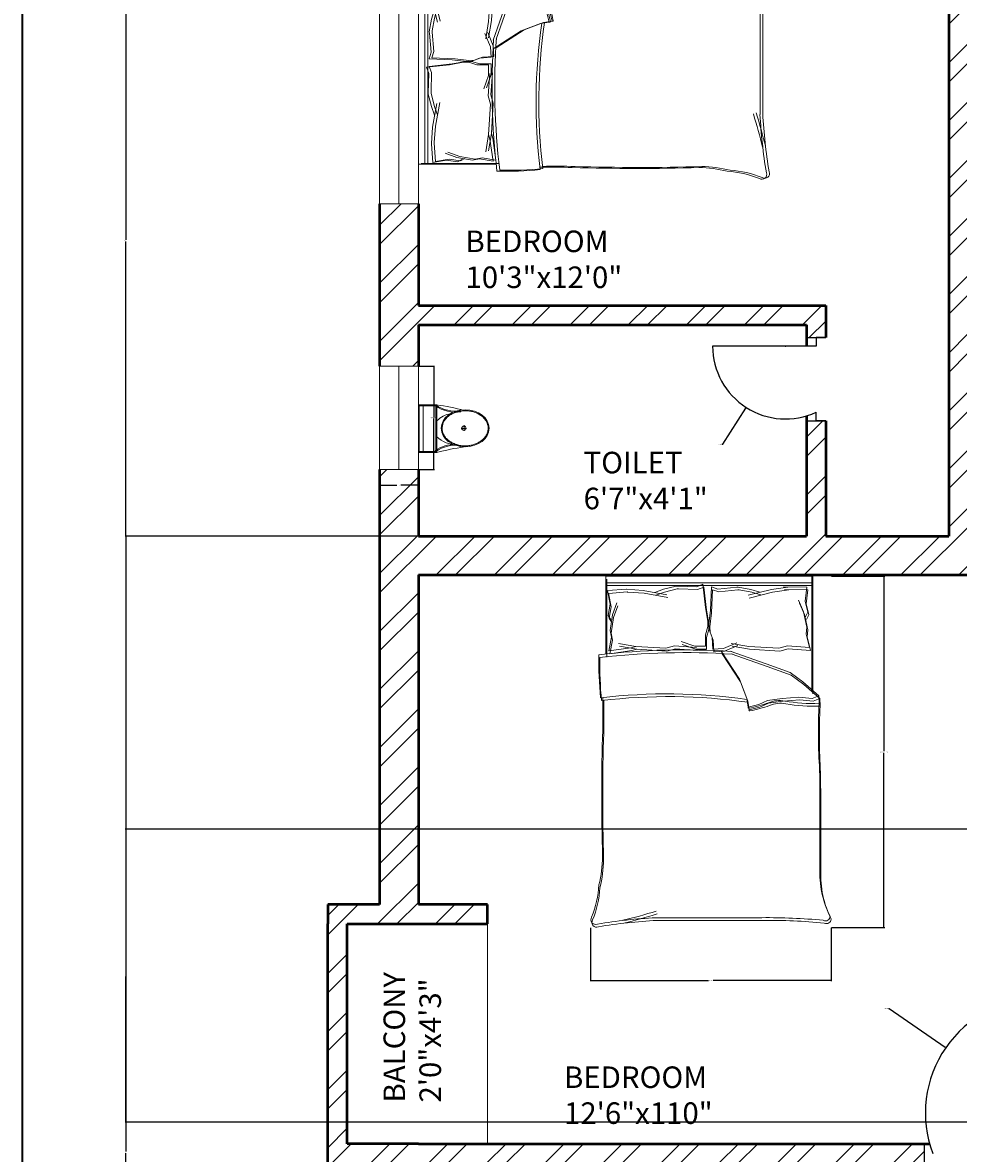
# Model space of a CAD drawing. Units: inches. Extents: x 1896 to 2572, y 1528 to 2474.
# Tile 6 of 10: x 1896 to 2113, y 2033 to 2295. Entities that reach past the tile are written whole.
import ezdxf

# ---------------------------------------------------------------- set-up
doc = ezdxf.new("R2010")
doc.units = ezdxf.units.IN
for name, color, linetype, lineweight in [('A-ANNO-DIMS', 2, 'Continuous', 18), ('A-ANNO-TTLB', 7, 'Continuous', 35), ('A-AREA-IDEN', 7, 'Continuous', 18), ('A-DOOR', 11, 'Continuous', 25), ('A-FLOR', 7, 'Continuous', 18), ('A-FLOR-FIXT', 8, 'Continuous', 18), ('A-FURN', 8, 'Continuous', 18), ('A-GLAZ', 131, 'Continuous', 20), ('A-WALL', 7, 'Continuous', 50)]:
    doc.layers.add(name, color=color, linetype=linetype, lineweight=lineweight)
doc.layers.add('A-WALL-PATT', color=215, linetype='Continuous', lineweight=13, true_color=0xa953a0)
doc.styles.get("Standard").update_dxf_attribs({"font": 'arial.ttf'})
doc.dimstyles.get("Standard").update_dxf_attribs({"dimtxt": 0.18, "dimasz": 0.18, "dimexe": 0.18, "dimexo": 0.0625, "dimgap": 0.09, "dimtad": 0, "dimtih": 1, "dimtoh": 1, "dimdec": 4, "dimzin": 0, "dimdsep": 46, "dimtxsty": 'Standard', "dimcen": 0.09, "dimadec": 0, "dimazin": 0, "dimtfac": 1, "dimtdec": 4, "dimtofl": 0, "dimtmove": 0, "dimatfit": 3, "dimfxl": 1, "dimtolj": 1, "dimtzin": 0, "dimarcsym": 0})

# ---------------------------------------------------------------- blocks, each defined once
blk = doc.blocks.new('A$C31115884')
for p, q in [((283, 498), (223, 498)), ((258, 466), (258, 523)), ((0, 200), (0, 0)), ((520, 200), (0, 200)), ((10, 190), (10, 10)), ((510, 190), (10, 190)), ((510, 10), (510, 190)), ((520, 0), (520, 200)), ((510, 54), (0, 54)), ((10, 10), (510, 10)), ((0, 0), (520, 0))]:
    blk.add_line(p, q)
blk.add_circle((256, 496), 23.6)
for centre, radius, start, end in [((2778, -205), 2807, 165.4549, 171.7133), ((3237, 905), 2807, 188.2867, 194.5451), ((-295, 403), 365, 324.2091, 9.3499), ((-295, 403), 375, 324.2091, 9.3499), ((139, 406), 293, 315.8436, 2.6563), ((806, 403), 375, 179.2036, 215.7909), ((806, 403), 365, 170.6501, 215.7909), ((384, 406), 293, 190.2774, 224.1564)]:
    blk.add_arc(centre, radius, start, end)
blk.add_ellipse((256, 510), major_axis=(0, -261), ratio=0.772727)
blk.add_open_spline([(256, 259), (263, 259), (270, 260), (288, 262), (299, 265), (320, 273), (330, 278), (350, 291), (360, 299), (378, 316), (386, 326), (402, 347), (409, 358), (421, 383), (427, 395), (436, 422), (440, 436), (445, 465), (447, 480), (448, 509), (448, 524), (445, 553), (443, 568), (436, 596), (432, 610), (422, 636), (416, 649), (402, 672), (395, 683), (379, 703), (370, 712), (351, 728), (341, 735), (321, 746), (310, 751), (289, 757), (278, 759), (256, 761), (245, 761), (223, 757), (212, 754), (191, 746), (181, 741), (161, 728), (151, 720), (133, 703), (125, 693), (110, 672), (103, 660), (90, 636), (85, 623), (76, 596), (72, 582), (67, 553), (66, 538), (64, 509), (65, 494), (68, 465), (70, 450), (77, 422), (81, 408), (91, 382), (97, 370), (111, 346), (118, 335), (135, 316), (144, 307), (162, 291), (172, 284), (193, 273), (203, 269), (225, 262), (236, 260), (250, 259), (253, 259), (256, 259)], degree=3, knots=[0, 0, 0, 0, 0.110105, 0.110105, 0.285049, 0.285049, 0.459994, 0.459994, 0.634938, 0.634938, 0.809882, 0.809882, 0.984827, 0.984827, 1.159771, 1.159771, 1.334715, 1.334715, 1.50966, 1.50966, 1.684604, 1.684604, 1.859549, 1.859549, 2.034493, 2.034493, 2.209437, 2.209437, 2.384382, 2.384382, 2.559326, 2.559326, 2.73427, 2.73427, 2.909215, 2.909215, 3.084159, 3.084159, 3.259103, 3.259103, 3.434048, 3.434048, 3.608992, 3.608992, 3.783936, 3.783936, 3.958881, 3.958881, 4.133825, 4.133825, 4.30877, 4.30877, 4.483714, 4.483714, 4.658658, 4.658658, 4.833603, 4.833603, 5.008547, 5.008547, 5.183491, 5.183491, 5.358436, 5.358436, 5.53338, 5.53338, 5.708324, 5.708324, 5.883269, 5.883269, 6.058213, 6.058213, 6.233158, 6.233158, 6.283185, 6.283185, 6.283185, 6.283185])
blk = doc.blocks.new('BED-DOUBLE')
for p, q in [((3.47, 63.33), (3.47, 81.44)), ((3.47, 63.33), (3.47, 81.44)), ((3.47, 81.44), (51.49, 81.44)), ((51.26, 81.44), (51.26, 54.83)), ((51.27, 81.44), (51.27, 54.83)), ((51.49, 81.44), (51.49, 80.8)), ((3.47, 79.91), (51.27, 79.91)), ((3.47, 79.91), (51.26, 79.91)), ((3.7, 62.69), (3.7, 80.8)), ((3.7, 62.69), (3.7, 80.8)), ((3.7, 79.27), (51.49, 79.27)), ((3.7, 79.27), (51.49, 79.27)), ((16.88, 78.42), (19.77, 79.14)), ((16.88, 78.42), (19.77, 79.14)), ((19.77, 79.14), (20.09, 79.14)), ((19.77, 79.14), (20.09, 79.14)), ((20.09, 79.14), (24.54, 78.99)), ((20.09, 79.14), (24.54, 78.99)), ((24.54, 78.99), (25.98, 79.57)), ((24.54, 78.99), (25.98, 79.57)), ((24.76, 78.36), (26.21, 78.93)), ((24.77, 78.36), (26.21, 78.93)), ((25.98, 79.57), (26.56, 74.22)), ((25.98, 79.57), (26.56, 74.22)), ((26.21, 78.93), (26.79, 73.58)), ((26.21, 78.93), (26.79, 73.58)), ((27.98, 78.95), (27.73, 73.58)), ((27.98, 78.95), (27.73, 73.58)), ((29.46, 78.46), (27.98, 78.95)), ((29.46, 78.46), (27.98, 78.95)), ((33.88, 78.89), (29.46, 78.46)), ((33.88, 78.89), (29.46, 78.46)), ((34.2, 78.91), (33.88, 78.89)), ((34.2, 78.91), (33.88, 78.89)), ((37.14, 78.37), (34.2, 78.91)), ((37.13, 78.37), (34.2, 78.91)), ((45.71, 78.9), (41.91, 78.37)), ((45.71, 78.9), (41.91, 78.37)), ((50.11, 78.89), (44.71, 78.98)), ((44.71, 78.98), (45.71, 78.9)), ((50.11, 78.89), (44.71, 78.98)), ((44.71, 78.98), (45.71, 78.9)), ((50.11, 78.89), (49.73, 75.68)), ((50.11, 78.89), (49.73, 75.68)), ((51.49, 80.8), (51.49, 54.19)), ((51.49, 80.8), (51.49, 54.19)), ((3.89, 78.13), (4.47, 74.95)), ((3.89, 78.13), (4.47, 74.95)), ((3.9, 78.11), (8.18, 78.43)), ((3.9, 78.11), (8.18, 78.43)), ((4.12, 77.49), (4.7, 74.31)), ((4.12, 77.49), (4.7, 74.31)), ((4.13, 77.47), (8.41, 77.8)), ((4.13, 77.47), (8.41, 77.8)), ((8.18, 78.43), (8.28, 78.42)), ((8.18, 78.43), (8.28, 78.42)), ((8.28, 78.42), (12.11, 78.13)), ((8.28, 78.42), (12.11, 78.13)), ((8.41, 77.8), (8.51, 77.78)), ((8.41, 77.8), (8.51, 77.78)), ((8.51, 77.78), (12.34, 77.49)), ((8.51, 77.78), (12.34, 77.49)), ((12.11, 78.13), (17.6, 77.12)), ((12.11, 78.13), (17.6, 77.12)), ((12.34, 77.49), (17.83, 76.48)), ((12.34, 77.49), (17.83, 76.48)), ((14.85, 77.69), (16.88, 78.42)), ((14.85, 77.69), (16.88, 78.42)), ((15.08, 77.05), (17.11, 77.78)), ((15.08, 77.05), (17.11, 77.78)), ((17.11, 77.78), (20, 78.5)), ((17.11, 77.78), (20, 78.5)), ((20, 78.5), (20.32, 78.5)), ((20, 78.5), (20.32, 78.5)), ((20.32, 78.5), (24.77, 78.36)), ((20.32, 78.5), (24.76, 78.36)), ((28.21, 78.31), (27.96, 72.94)), ((28.2, 78.31), (27.96, 72.94)), ((29.68, 77.83), (28.2, 78.31)), ((29.68, 77.83), (28.21, 78.31)), ((34.11, 78.25), (29.68, 77.83)), ((34.11, 78.25), (29.68, 77.83)), ((34.43, 78.27), (34.11, 78.25)), ((34.43, 78.27), (34.11, 78.25)), ((37.36, 77.73), (34.43, 78.27)), ((37.36, 77.73), (34.43, 78.27)), ((41.91, 78.37), (36.49, 77.02)), ((41.91, 78.37), (36.49, 77.02)), ((42.14, 77.73), (36.72, 76.38)), ((42.14, 77.73), (36.72, 76.38)), ((39.2, 77.77), (37.13, 78.37)), ((39.2, 77.77), (37.14, 78.37)), ((39.43, 77.13), (37.36, 77.73)), ((39.43, 77.13), (37.36, 77.73)), ((45.94, 78.26), (42.14, 77.73)), ((45.94, 78.26), (42.14, 77.73)), ((50.34, 78.25), (44.94, 78.34)), ((44.94, 78.34), (45.94, 78.26)), ((50.34, 78.25), (44.94, 78.34)), ((44.94, 78.34), (45.94, 78.26)), ((50.34, 78.25), (49.96, 75.04)), ((50.34, 78.25), (49.96, 75.04)), ((4.47, 74.95), (4.04, 72.34)), ((4.47, 74.95), (4.04, 72.34)), ((4.7, 74.31), (4.27, 71.7)), ((4.7, 74.31), (4.27, 71.7)), ((5.05, 72.49), (6.06, 75.24)), ((5.05, 72.49), (6.06, 75.24)), ((5.28, 71.85), (6.29, 74.6)), ((5.28, 71.85), (6.29, 74.6)), ((26.56, 74.22), (27.14, 71.04)), ((26.56, 74.22), (27.14, 71.04)), ((26.79, 73.58), (27.37, 70.4)), ((26.79, 73.58), (27.37, 70.4)), ((27.73, 73.58), (27.35, 70.37)), ((27.73, 73.58), (27.35, 70.37)), ((49.31, 73.19), (48.13, 75.87)), ((49.31, 73.19), (48.13, 75.87)), ((49.54, 72.55), (48.36, 75.23)), ((49.54, 72.55), (48.36, 75.23)), ((49.73, 75.68), (50.33, 73.11)), ((49.73, 75.68), (50.33, 73.11)), ((49.96, 75.04), (50.56, 72.47)), ((49.96, 75.04), (50.56, 72.47)), ((4.04, 72.34), (4.62, 71.33)), ((4.04, 72.34), (4.62, 71.33)), ((4.27, 71.7), (4.85, 70.69)), ((4.27, 71.7), (4.85, 70.69)), ((4.47, 68.87), (5.05, 72.49)), ((4.47, 68.87), (5.05, 72.49)), ((4.7, 68.23), (5.28, 71.85)), ((4.7, 68.23), (5.28, 71.85)), ((27.14, 71.04), (27.14, 69.74)), ((27.14, 71.04), (27.14, 69.74)), ((27.96, 72.94), (27.58, 69.73)), ((27.96, 72.94), (27.58, 69.73)), ((50.11, 69.61), (49.31, 73.19)), ((50.11, 69.61), (49.31, 73.19)), ((50.34, 68.98), (49.54, 72.55)), ((50.34, 68.98), (49.54, 72.55)), ((50.33, 73.11), (49.81, 72.06)), ((50.33, 73.11), (49.81, 72.06)), ((50.56, 72.47), (50.04, 71.42)), ((50.56, 72.47), (50.04, 71.42)), ((4.76, 67.28), (4.47, 68.87)), ((4.76, 67.28), (4.47, 68.87)), ((4.99, 66.64), (4.7, 68.23)), ((4.99, 66.64), (4.7, 68.23)), ((27.14, 69.74), (26.56, 67.86)), ((27.14, 69.74), (26.56, 67.86)), ((27.37, 69.1), (26.79, 67.22)), ((27.37, 69.1), (26.79, 67.22)), ((27.35, 70.37), (27.44, 69.07)), ((27.35, 70.37), (27.44, 69.07)), ((27.37, 70.4), (27.37, 69.1)), ((27.37, 70.4), (27.37, 69.1)), ((27.44, 69.07), (28.13, 67.23)), ((27.44, 69.07), (28.13, 67.23)), ((27.58, 69.73), (27.66, 68.43)), ((27.58, 69.73), (27.66, 68.43)), ((27.66, 68.43), (28.36, 66.59)), ((27.66, 68.43), (28.36, 66.59)), ((49.92, 68.01), (50.11, 69.61)), ((49.92, 68.01), (50.11, 69.61)), ((50.15, 67.37), (50.34, 68.98)), ((50.15, 67.37), (50.34, 68.98)), ((4.18, 64.1), (4.76, 67.28)), ((4.18, 64.1), (4.76, 67.28)), ((4.41, 63.46), (4.99, 66.64)), ((4.41, 63.46), (4.99, 66.64)), ((6.38, 65.81), (10.41, 65.15)), ((6.38, 65.81), (10.41, 65.15)), ((24.1, 65.18), (20.96, 66.27)), ((24.1, 65.18), (20.96, 66.27)), ((24.33, 64.54), (21.19, 65.63)), ((24.33, 64.54), (21.19, 65.63)), ((26.56, 67.86), (26.56, 65.18)), ((26.56, 67.86), (26.56, 65.18)), ((26.79, 67.22), (26.79, 64.54)), ((26.79, 67.22), (26.79, 64.54)), ((28.13, 67.23), (28.3, 64.55)), ((28.13, 67.23), (28.3, 64.55)), ((28.36, 66.59), (28.53, 63.91)), ((28.36, 66.59), (28.53, 63.91)), ((30.75, 64.7), (33.82, 65.99)), ((30.75, 64.7), (33.82, 65.99)), ((32.56, 65.81), (36.6, 65.15)), ((32.56, 65.81), (36.6, 65.15)), ((50.7, 64.87), (49.92, 68.01)), ((50.7, 64.87), (49.92, 68.01)), ((50.93, 64.23), (50.15, 67.37)), ((50.93, 64.23), (50.15, 67.37)), ((9.28, 64.83), (4.18, 64.1)), ((9.28, 64.83), (4.18, 64.1)), ((9.51, 64.19), (4.41, 63.46)), ((9.51, 64.19), (4.41, 63.46)), ((6.61, 65.18), (10.64, 64.51)), ((6.61, 65.18), (10.64, 64.51)), ((10.41, 65.15), (9.28, 64.83)), ((10.41, 65.15), (9.28, 64.83)), ((10.64, 64.51), (9.51, 64.19)), ((10.64, 64.51), (9.51, 64.19)), ((10.41, 65.15), (17.42, 64.72)), ((10.41, 65.15), (17.42, 64.72)), ((10.64, 64.51), (17.65, 64.08)), ((10.64, 64.51), (17.65, 64.08)), ((17.42, 64.72), (19.38, 65.27)), ((17.42, 64.72), (19.38, 65.27)), ((17.65, 64.08), (19.61, 64.63)), ((17.65, 64.08), (19.61, 64.63)), ((19.38, 65.27), (24.52, 64.87)), ((19.38, 65.27), (24.52, 64.87)), ((19.61, 64.63), (24.74, 64.23)), ((19.61, 64.63), (24.74, 64.23)), ((26.56, 65.18), (24.1, 65.18)), ((26.56, 65.18), (24.1, 65.18)), ((26.79, 64.54), (24.33, 64.54)), ((26.79, 64.54), (24.33, 64.54)), ((28.3, 64.55), (30.75, 64.7)), ((28.3, 64.55), (30.75, 64.7)), ((28.53, 63.91), (30.98, 64.06)), ((28.53, 63.91), (30.98, 64.06)), ((30.26, 64.06), (34.45, 57.57)), ((30.26, 64.06), (34.45, 57.57)), ((30.49, 63.42), (34.68, 56.93)), ((30.49, 63.42), (34.68, 56.93)), ((30.98, 64.06), (34.05, 65.35)), ((30.98, 64.06), (34.05, 65.35)), ((40.64, 61.13), (32.31, 64.06)), ((40.64, 61.13), (32.31, 64.06)), ((40.87, 60.49), (32.53, 63.42)), ((40.87, 60.49), (32.53, 63.42)), ((32.79, 65.18), (36.82, 64.51)), ((32.79, 65.18), (36.82, 64.51)), ((36.6, 65.15), (43.61, 64.72)), ((36.6, 65.15), (43.61, 64.72)), ((36.82, 64.51), (43.83, 64.08)), ((36.82, 64.51), (43.83, 64.08)), ((43.61, 64.72), (45.57, 65.27)), ((43.61, 64.72), (45.57, 65.27)), ((43.83, 64.08), (45.79, 64.63)), ((43.83, 64.08), (45.79, 64.63)), ((45.57, 65.27), (50.7, 64.87)), ((45.57, 65.27), (50.7, 64.87)), ((45.79, 64.63), (50.93, 64.23)), ((45.79, 64.63), (50.93, 64.23)), ((46.22, 59.11), (40.64, 61.13)), ((46.22, 59.11), (40.64, 61.13)), ((46.45, 58.48), (40.87, 60.49)), ((46.45, 58.48), (40.87, 60.49)), ((49.16, 56.95), (46.22, 59.11)), ((49.16, 56.95), (46.22, 59.11)), ((49.39, 56.31), (46.45, 58.48)), ((49.39, 56.31), (46.45, 58.48)), ((34.45, 57.57), (36.15, 53.08)), ((34.45, 57.57), (36.15, 53.08)), ((34.68, 56.93), (36.38, 52.44)), ((34.68, 56.93), (36.38, 52.44)), ((52.87, 53.7), (49.16, 56.95)), ((52.87, 53.7), (49.16, 56.95)), ((53.1, 53.06), (49.39, 56.31)), ((53.1, 53.06), (49.39, 56.31)), ((36.15, 53.08), (36.46, 51.07)), ((36.15, 53.08), (36.46, 51.07)), ((38.94, 51.69), (40.95, 52.61)), ((38.94, 51.69), (40.95, 52.61)), ((40.95, 52.61), (44.36, 53.08)), ((40.95, 52.61), (44.36, 53.08)), ((44.36, 53.08), (48.23, 53.39)), ((44.36, 53.08), (48.23, 53.39)), ((44.59, 52.44), (48.46, 52.75)), ((44.59, 52.44), (48.46, 52.75)), ((48.23, 53.39), (51.33, 53.08)), ((48.23, 53.39), (51.33, 53.08)), ((48.46, 52.75), (51.56, 52.44)), ((48.46, 52.75), (51.56, 52.44)), ((51.33, 53.08), (52.87, 53.7)), ((51.33, 53.08), (52.87, 53.7)), ((51.56, 52.44), (53.1, 53.06)), ((51.56, 52.44), (53.1, 53.06)), ((52.95, 51.95), (52.87, 53.7, 3.87)), ((52.95, 51.95), (52.87, 53.7, 3.87)), ((53.18, 51.31), (53.1, 53.06, 3.87)), ((53.17, 51.31), (53.1, 53.06, 3.87)), ((36.38, 52.44), (36.69, 50.43)), ((36.38, 52.44), (36.69, 50.43)), ((36.46, 51.07), (38.94, 51.69)), ((36.46, 51.07), (38.94, 51.69)), ((36.69, 50.43), (39.17, 51.05)), ((36.69, 50.43), (39.17, 51.05)), ((39.17, 51.05), (41.18, 51.97)), ((39.17, 51.05), (41.18, 51.97)), ((41.18, 51.97), (44.59, 52.44)), ((41.18, 51.97), (44.59, 52.44)), ((15.06, 2.2), (39.68, 2.2)), ((15.06, 2.2), (39.68, 2.2)), ((15.29, 1.56), (39.91, 1.56)), ((15.29, 1.56), (39.91, 1.56))]:
    blk.add_line(p, q)
for centre, radius, start, end in [((85.16, 61.35), 83.31, 178.7218, 185.604), ((85.16, 61.35), 83.31, 178.7218, 185.604), ((21.36, -100.61), 164.97, 86.0865, 96.7821), ((21.36, -100.61), 164.97, 86.0865, 96.7821), ((21.59, -101.25), 164.97, 86.0865, 96.7821), ((21.59, -101.25), 164.97, 86.0865, 96.7821), ((85.39, 60.71), 83.31, 178.7218, 185.604), ((85.39, 60.71), 83.31, 178.7218, 185.604), ((17.76, -74.87), 129.02, 81.7845, 96.9006), ((17.76, -74.87), 129.02, 81.7845, 96.9006), ((17.98, -75.51), 129.02, 81.7845, 96.9006), ((17.98, -75.51), 129.02, 81.7845, 96.9006), ((-167.31, 50.27), 170.11, 358.4762, 1.0082), ((-167.31, 50.27), 170.11, 358.4762, 1.0082), ((-167.08, 49.63), 170.11, 358.4762, 1.0082), ((-167.08, 49.63), 170.11, 358.4762, 1.0082), ((43.74, 46.38), 6.22, 78.6608, 113.7384), ((43.74, 46.38), 6.22, 78.6608, 113.7384), ((36.64, 51), 0.185, 160.2464, 271.1377), ((36.64, 51), 0.185, 160.2464, 271.1377), ((31.15, 79.96), 29.65, 280.6617, 289.8806), ((31.15, 79.96), 29.65, 280.6617, 289.8806), ((36.86, 50.36), 0.185, 160.2464, 271.1377), ((36.86, 50.36), 0.185, 160.2464, 271.1377), ((31.38, 79.32), 29.65, 280.6617, 289.8806), ((31.38, 79.32), 29.65, 280.6617, 289.8806), ((43.97, 45.74), 6.22, 78.6608, 113.7384), ((43.97, 45.74), 6.22, 78.6608, 113.7384), ((51.33, 88.1), 36.18, 259.8763, 272.5657), ((51.33, 88.1), 36.18, 259.8763, 272.5657), ((51.56, 87.46), 36.18, 259.8763, 272.5657), ((51.56, 87.46), 36.18, 259.8763, 272.5657), ((182.27, 45.13), 129.5, 176.9791, 183.8365), ((182.27, 45.13), 129.5, 176.9791, 183.8365), ((182.49, 44.49), 129.5, 176.9791, 183.8365), ((182.49, 44.49), 129.5, 176.9791, 183.8365), ((484.82, 30.83), 482.31, 178.2277, 181.7185), ((484.82, 30.83), 482.31, 178.2277, 181.7185), ((485.05, 30.19), 482.31, 178.2277, 181.7185), ((485.05, 30.19), 482.31, 178.2277, 181.7185), ((-4508.74, 13.62), 4561.86, 0.00217, 0.28689), ((-4508.74, 13.62), 4561.86, 0.00217, 0.28689), ((-4508.52, 12.98), 4561.86, 0.00217, 0.28689), ((-4508.52, 12.98), 4561.86, 0.00217, 0.28689), ((-26.9, 16.93), 29.63, 346.0648, 358.9113), ((-26.9, 16.93), 29.63, 346.0648, 358.9113), ((-26.67, 16.29), 29.63, 346.0648, 358.9113), ((-26.67, 16.29), 29.63, 346.0648, 358.9113), ((76.16, 12.78), 23.07, 177.4714, 206.4681), ((76.16, 12.78), 23.07, 177.4714, 206.4681), ((76.39, 12.14), 23.07, 177.4714, 206.4681), ((76.39, 12.14), 23.07, 177.4714, 206.4681), ((-21.66, 11.17), 23.56, 337.9751, 356.652), ((-21.66, 11.17), 23.56, 337.9751, 356.652), ((-21.43, 10.53), 23.56, 337.9751, 356.652), ((-21.43, 10.53), 23.56, 337.9751, 356.652), ((-17.22, 105.16), 106.46, 283.3832, 287.7053), ((-17.22, 105.16), 106.46, 283.3832, 287.7053), ((-16.99, 104.52), 106.46, 283.3832, 287.7053), ((-16.99, 104.52), 106.46, 283.3832, 287.7053), ((1.09, 1.73), 1.09, 146.1736, 293.4781), ((1.09, 1.73), 1.09, 146.1736, 293.4781), ((1.32, 1.09), 1.09, 146.1736, 293.4781), ((1.32, 1.09), 1.09, 146.1736, 293.4781), ((21.43, -119.39), 121.76, 92.9958, 99.4091), ((21.43, -119.39), 121.76, 92.9958, 99.4091), ((21.65, -120.03), 121.76, 92.9958, 99.4091), ((21.65, -120.03), 121.76, 92.9958, 99.4091), ((41.15, -130.83), 133.04, 84.4998, 90.6351), ((41.15, -130.83), 133.04, 84.4998, 90.6351), ((41.38, -131.47), 133.04, 84.4998, 90.6351), ((41.38, -131.47), 133.04, 84.4998, 90.6351), ((54.41, 2.57), 1.1, 242.6588, 356.02), ((54.41, 2.57), 1.1, 242.6588, 356.02), ((54.64, 1.93), 1.1, 242.6588, 356.02), ((54.64, 1.93), 1.1, 242.6588, 356.02)]:
    blk.add_arc(centre, radius, start, end)
blk = doc.blocks.new('WIN-24IN')
for p, q in [((4.5, 24), (0, 24)), ((0, 24), (9, 24)), ((0, 24), (0, 0)), ((4.5, 0), (4.5, 24)), ((9, 0), (9, 24)), ((0, 0), (9, 0)), ((9, 0), (4.5, 0))]:
    blk.add_line(p, q)
blk = doc.blocks.new('WIN-60IN')
for p, q in [((4.5, 60), (0, 60)), ((0, 60), (9, 60)), ((0, 60), (0, 0)), ((4.5, 0), (4.5, 60)), ((9, 0), (9, 60)), ((0, 0), (9, 0)), ((9, 0), (4.5, 0))]:
    blk.add_line(p, q)
blk = doc.blocks.new('*D7')
at = {"layer": 'A-ANNO-DIMS', "color": 0, "lineweight": -2, "transparency": 16777216}
for p, q in [((1987.68, 2215.35), (1991.4, 2215.35)), ((1991.22, 2215.17), (1991.22, 2203.53)), ((1991.22, 2191.53), (1991.22, 2203.17)), ((1987.68, 2191.35), (1991.4, 2191.35))]:
    blk.add_line(p, q, dxfattribs=at)
at = {"layer": 'A-ANNO-DIMS', "color": 0, "transparency": 16777216}
for points in [[(1991.19, 2215.17), (1991.25, 2215.17), (1991.22, 2215.35)], [(1991.19, 2191.53), (1991.25, 2191.53), (1991.22, 2191.35)]]:
    blk.add_solid(points, dxfattribs=at)
at = {"layer": 'Defpoints', "color": 0, "transparency": 16777216}
for p in [(1987.62, 2215.35), (1991.22, 2215.35), (1987.62, 2191.35)]:
    blk.add_point(p, dxfattribs=at)
at = {"layer": 'A-ANNO-DIMS', "color": 0, "transparency": 16777216, "insert": (1991.22, 2203.35), "char_height": 0.18, "attachment_point": 5}
blk.add_mtext('\\A1;WDW 24 TYP.', dxfattribs=at)
blk = doc.blocks.new('*D8')
at = {"layer": 'A-ANNO-DIMS', "color": 0, "lineweight": -2, "transparency": 16777216}
for p, q in [((1978.62, 2191.29), (1978.62, 2187.57)), ((1987.62, 2191.29), (1987.62, 2187.57)), ((1978.8, 2187.75), (1982.66, 2187.75)), ((1987.44, 2187.75), (1983.58, 2187.75))]:
    blk.add_line(p, q, dxfattribs=at)
at = {"layer": 'A-ANNO-DIMS', "color": 0, "transparency": 16777216}
for points in [[(1978.8, 2187.78), (1978.8, 2187.72), (1978.62, 2187.75)], [(1987.44, 2187.78), (1987.44, 2187.72), (1987.62, 2187.75)]]:
    blk.add_solid(points, dxfattribs=at)
at = {"layer": 'Defpoints', "color": 0, "transparency": 16777216}
for p in [(1978.62, 2191.35), (1987.62, 2191.35), (1987.62, 2187.75)]:
    blk.add_point(p, dxfattribs=at)
at = {"layer": 'A-ANNO-DIMS', "color": 0, "transparency": 16777216, "insert": (1983.12, 2187.75), "char_height": 0.18, "attachment_point": 5}
blk.add_mtext('\\A1;9 TYP.', dxfattribs=at)
blk = doc.blocks.new('*D11')
at = {"layer": 'A-ANNO-DIMS', "color": 0, "lineweight": -2, "transparency": 16777216}
for p, q in [((2083.44, 2166.59), (2095.78, 2166.59)), ((2095.6, 2166.41), (2095.6, 2125.99)), ((2095.6, 2085.22), (2095.6, 2125.63)), ((2083.44, 2085.04), (2095.78, 2085.04))]:
    blk.add_line(p, q, dxfattribs=at)
at = {"layer": 'A-ANNO-DIMS', "color": 0, "transparency": 16777216}
for points in [[(2095.57, 2166.41), (2095.63, 2166.41), (2095.6, 2166.59)], [(2095.57, 2085.22), (2095.63, 2085.22), (2095.6, 2085.04)]]:
    blk.add_solid(points, dxfattribs=at)
at = {"layer": 'Defpoints', "color": 0, "transparency": 16777216}
for p in [(2083.37, 2166.59), (2095.6, 2166.59), (2083.37, 2085.04)]:
    blk.add_point(p, dxfattribs=at)
at = {"layer": 'A-ANNO-DIMS', "color": 0, "transparency": 16777216, "insert": (2095.6, 2125.81), "char_height": 0.18, "attachment_point": 5}
blk.add_mtext('\\A1;DOUBLE BED 82 TYP.', dxfattribs=at)
blk = doc.blocks.new('*D12')
at = {"layer": 'A-ANNO-DIMS', "color": 0, "lineweight": -2, "transparency": 16777216}
for p, q in [((2027.55, 2084.97), (2027.55, 2072.62)), ((2083.37, 2084.97), (2083.37, 2072.62)), ((2027.73, 2072.8), (2054.93, 2072.8)), ((2083.19, 2072.8), (2055.99, 2072.8))]:
    blk.add_line(p, q, dxfattribs=at)
at = {"layer": 'A-ANNO-DIMS', "color": 0, "transparency": 16777216}
for points in [[(2027.73, 2072.83), (2027.73, 2072.77), (2027.55, 2072.8)], [(2083.19, 2072.83), (2083.19, 2072.77), (2083.37, 2072.8)]]:
    blk.add_solid(points, dxfattribs=at)
at = {"layer": 'Defpoints', "color": 0, "transparency": 16777216}
for p in [(2027.55, 2085.04), (2083.37, 2085.04), (2083.37, 2072.8)]:
    blk.add_point(p, dxfattribs=at)
at = {"layer": 'A-ANNO-DIMS', "color": 0, "transparency": 16777216, "insert": (2055.46, 2072.8), "char_height": 0.18, "attachment_point": 5}
blk.add_mtext('\\A1;56 TYP.', dxfattribs=at)
blk = doc.blocks.new('*D26')
at = {"layer": 'A-ANNO-DIMS', "color": 0, "lineweight": -2, "transparency": 16777216}
for p, q in [((1978.56, 2313.03), (1919.59, 2313.03)), ((1919.77, 2312.85), (1919.77, 2244.65)), ((1919.77, 2176.08), (1919.77, 2244.28)), ((1987.56, 2175.9), (1919.59, 2175.9))]:
    blk.add_line(p, q, dxfattribs=at)
at = {"layer": 'A-ANNO-DIMS', "color": 0, "transparency": 16777216}
for points in [[(1919.74, 2312.85), (1919.8, 2312.85), (1919.77, 2313.03)], [(1919.74, 2176.08), (1919.8, 2176.08), (1919.77, 2175.9)]]:
    blk.add_solid(points, dxfattribs=at)
at = {"layer": 'Defpoints', "color": 0, "transparency": 16777216}
for p in [(1978.62, 2313.03), (1919.77, 2175.9), (1987.62, 2175.9)]:
    blk.add_point(p, dxfattribs=at)
at = {"layer": 'A-ANNO-DIMS', "color": 0, "transparency": 16777216, "insert": (1919.77, 2244.47), "char_height": 0.18, "attachment_point": 5}
blk.add_mtext('\\A1;137.14', dxfattribs=at)
blk = doc.blocks.new('*D27')
at = {"layer": 'A-ANNO-DIMS', "color": 0, "lineweight": -2, "transparency": 16777216}
for p, q in [((1987.56, 2175.9), (1919.59, 2175.9)), ((1919.77, 2175.72), (1919.77, 2033.08)), ((1919.77, 1890.08), (1919.77, 2032.72)), ((1987.56, 1889.9), (1919.59, 1889.9))]:
    blk.add_line(p, q, dxfattribs=at)
at = {"layer": 'A-ANNO-DIMS', "color": 0, "transparency": 16777216}
for points in [[(1919.74, 2175.72), (1919.8, 2175.72), (1919.77, 2175.9)], [(1919.74, 1890.08), (1919.8, 1890.08), (1919.77, 1889.9)]]:
    blk.add_solid(points, dxfattribs=at)
at = {"layer": 'Defpoints', "color": 0, "transparency": 16777216}
for p in [(1987.62, 2175.9), (1919.77, 1889.9), (1987.62, 1889.9)]:
    blk.add_point(p, dxfattribs=at)
at = {"layer": 'A-ANNO-DIMS', "color": 0, "transparency": 16777216, "insert": (1919.77, 2032.9), "char_height": 0.18, "attachment_point": 5}
blk.add_mtext('\\A1;286', dxfattribs=at)
blk = doc.blocks.new('*D30')
at = {"layer": 'A-ANNO-DIMS', "color": 0, "lineweight": -2, "transparency": 16777216}
for p, q in [((2347.56, 2107.9), (1919.59, 2107.9)), ((1919.77, 2107.72), (1919.77, 2074.08)), ((1919.77, 2040.08), (1919.77, 2073.72)), ((2347.56, 2039.9), (1919.59, 2039.9))]:
    blk.add_line(p, q, dxfattribs=at)
at = {"layer": 'A-ANNO-DIMS', "color": 0, "transparency": 16777216}
for points in [[(1919.74, 2107.72), (1919.8, 2107.72), (1919.77, 2107.9)], [(1919.74, 2040.08), (1919.8, 2040.08), (1919.77, 2039.9)]]:
    blk.add_solid(points, dxfattribs=at)
at = {"layer": 'Defpoints', "color": 0, "transparency": 16777216}
for p in [(1919.77, 2107.9), (2347.62, 2107.9), (2347.62, 2039.9)]:
    blk.add_point(p, dxfattribs=at)
at = {"layer": 'A-ANNO-DIMS', "color": 0, "transparency": 16777216, "insert": (1919.77, 2073.9), "char_height": 0.18, "attachment_point": 5}
blk.add_mtext('\\A1;68', dxfattribs=at)
blk = doc.blocks.new('*D43')
at = {"layer": 'A-ANNO-DIMS', "color": 0, "lineweight": -2, "transparency": 16777216}
for p, q in [((2096.63, 2066.26), (2096.81, 2066.26)), ((2096.81, 2066.26), (2109.79, 2057.28)), ((2131.74, 2042.03), (2131.92, 2042.03)), ((2131.83, 2041.94), (2131.83, 2042.12))]:
    blk.add_line(p, q, dxfattribs=at)
at = {"layer": 'A-ANNO-DIMS', "color": 0, "transparency": 16777216}
blk.add_solid([(2109.81, 2057.3), (2109.78, 2057.25), (2109.94, 2057.18)], dxfattribs=at)
at = {"layer": 'Defpoints', "color": 0, "transparency": 16777216}
for p in [(2109.94, 2057.18), (2131.83, 2042.03)]:
    blk.add_point(p, dxfattribs=at)
at = {"layer": 'A-ANNO-DIMS', "color": 0, "transparency": 16777216, "insert": (2096.15, 2066.26), "char_height": 0.18, "attachment_point": 5}
blk.add_mtext('\\A1;R26.62', dxfattribs=at)
blk = doc.blocks.new('*D51')
at = {"layer": 'A-ANNO-DIMS', "color": 0, "lineweight": -2, "transparency": 16777216}
for p, q in [((2072.78, 2219.9), (2072.78, 2220.08)), ((2072.69, 2219.99), (2072.87, 2219.99)), ((2058.21, 2197.2), (2063.58, 2205.59)), ((2058.03, 2197.2), (2058.21, 2197.2))]:
    blk.add_line(p, q, dxfattribs=at)
at = {"layer": 'A-ANNO-DIMS', "color": 0, "transparency": 16777216}
blk.add_solid([(2063.55, 2205.61), (2063.6, 2205.58), (2063.67, 2205.74)], dxfattribs=at)
at = {"layer": 'Defpoints', "color": 0, "transparency": 16777216}
for p in [(2072.78, 2219.99), (2063.67, 2205.74)]:
    blk.add_point(p, dxfattribs=at)
at = {"layer": 'A-ANNO-DIMS', "color": 0, "transparency": 16777216, "insert": (2057.48, 2197.2), "char_height": 0.18, "attachment_point": 5}
blk.add_mtext('\\A1;R16.903', dxfattribs=at)

msp = doc.modelspace()

# ---------------------------------------------------------------- hatches: boundary and pattern name
at = {"layer": 'A-WALL-PATT'}
h = msp.add_hatch(dxfattribs=at)
h.set_pattern_fill('ANSI32', color=256)
h.paths.add_polyline_path([(2071.6224, 2382.3979), (2071.6224, 2422.3979), (2110.6224, 2422.3979), (2110.6224, 2382.3979), (2110.6224, 2357.5961), (2119.6224, 2357.5961), (2119.6224, 2422.3979), (2171.6224, 2422.3979), (2171.6224, 2373.3979), (2193.5093, 2373.3979), (2193.5093, 2377.8979), (2193.5093, 2382.3979), (2180.6224, 2382.3979), (2180.6224, 2431.3979), (2171.6224, 2431.3979), (2119.6224, 2431.3979), (2110.6224, 2431.3979), (2062.6224, 2431.3979), (2062.6224, 2422.3979), (2062.6224, 2382.3979), (1978.6224, 2382.3979), (1978.6224, 2313.0337), (1987.6224, 2313.0337), (1987.6224, 2373.3979), (2062.6224, 2373.3979), (2067.1224, 2373.3979), (2067.1224, 2353.7982), (2071.6224, 2353.8883)])
h.paths.add_polyline_path([(2287.4624, 2382.3979), (2229.5093, 2382.3979), (2229.5093, 2373.3979), (2253.1224, 2373.3979), (2253.1224, 2175.8979), (2247.1039, 2175.8979), (2247.1039, 2166.8979), (2253.1224, 2166.8979), (2253.1224, 2150.8283), (2262.1224, 2150.8283), (2262.1224, 2166.8979), (2262.1224, 2236.8979), (2349.0731, 2236.8979), (2349.0731, 2239.1479), (2349.0731, 2241.3979), (2262.1224, 2241.3979), (2262.1224, 2373.3979), (2287.4624, 2373.3979)])
h.paths.add_polyline_path([(2452.6224, 2382.3979), (2347.4624, 2382.3979), (2347.4624, 2373.3979), (2382.1224, 2373.3979), (2382.1224, 2334.0335), (2386.6224, 2334.0335), (2386.6224, 2373.3979), (2443.6224, 2373.3979), (2443.6224, 2316.2056), (2452.6224, 2316.2056)])
h.paths.add_polyline_path([(2452.6224, 2292.2056), (2448.1224, 2292.2056), (2443.6224, 2292.2056), (2443.6224, 2292.0047), (2443.6224, 2280.9372), (2443.6224, 2268.3979), (2386.6224, 2268.3979), (2386.6224, 2312.4044), (2384.3724, 2312.4044), (2382.1224, 2312.4044), (2382.1224, 2241.3979), (2379.1336, 2241.3979), (2379.1336, 2236.8979), (2386.6224, 2236.8979), (2386.6224, 2263.8979), (2443.6224, 2263.8979), (2443.6224, 2248.8449), (2452.6224, 2248.8449)])
h.paths.add_polyline_path([(2364.1285, 2116.8979), (2262.1224, 2116.8979), (2262.1224, 2120.5401), (2257.6224, 2120.5401), (2253.1224, 2120.5401), (2253.1224, 2107.8979), (2262.1224, 2107.8979), (2269.354, 2107.8979), (2269.354, 2094.0702), (2278.354, 2094.0702), (2278.354, 2107.8979), (2347.6224, 2107.8979), (2347.6224, 2039.8979), (2278.354, 2039.8979), (2278.354, 2054.7605), (2269.354, 2054.7605), (2269.354, 2030.8979), (2278.354, 2030.8979), (2443.6224, 2030.8979), (2443.6224, 2015.198), (2452.6224, 2015.198), (2452.6224, 2030.8979), (2464.6224, 2030.8979), (2469.1224, 2030.8979), (2469.1224, 2117.0352), (2452.6767, 2116.9466), (2452.6285, 2125.8979), (2452.6224, 2125.8979), (2452.6224, 2212.8449), (2443.6224, 2212.8449), (2443.6224, 2116.8979), (2385.832, 2116.8979), (2385.832, 2112.3979), (2385.832, 2107.8979), (2464.6224, 2107.8979), (2464.6224, 2039.8979), (2443.6224, 2039.8979), (2356.6224, 2039.8979), (2356.6224, 2107.8979), (2364.1285, 2107.8979)])
h.paths.add_polyline_path([(2452.6224, 1967.198), (2443.6224, 1967.198), (2443.6224, 1955.8979), (2259.1224, 1955.8979), (2254.6224, 1955.8979), (2254.6224, 1941.6358), (2263.6224, 1941.6358), (2263.6224, 1946.8979), (2379.1224, 1946.8979), (2379.1224, 1913.0204), (2383.6224, 1913.0204), (2383.6224, 1946.8979), (2443.6224, 1946.8979), (2443.6224, 1930.729), (2452.6224, 1930.729)])
h.paths.add_polyline_path([(2469.1224, 1871.8979), (2464.6224, 1871.8979), (2452.6224, 1871.8979), (2452.6224, 1894.729), (2443.6224, 1894.729), (2443.6224, 1871.8979), (2388.1304, 1871.8979), (2388.1304, 1867.3979), (2443.6224, 1867.3979), (2464.6224, 1867.3979), (2464.6224, 1817.8979), (2443.6224, 1817.8979), (2388.1304, 1817.8979), (2388.1304, 1815.6479), (2388.1304, 1813.3979), (2391.1224, 1813.3979), (2391.1224, 1747.8899), (2395.6224, 1747.8899), (2395.6224, 1813.3979), (2443.6224, 1813.3979), (2443.6224, 1781.4434), (2452.6224, 1781.4434), (2452.6224, 1813.3979), (2464.6224, 1813.3979), (2469.1224, 1813.3979)])
h.paths.add_polyline_path([(2263.6224, 1910.9737), (2259.1224, 1910.9737), (2254.6224, 1910.9737), (2254.6224, 1889.8979), (2251.2778, 1889.8979), (2251.2778, 1880.8979), (2254.6224, 1880.8979), (2254.6224, 1817.8979), (2254.6224, 1754.8979), (2254.6224, 1693.3979), (2254.6224, 1684.3979), (2254.6224, 1672.3979), (2200.6224, 1672.3979), (2200.6224, 1684.3979), (2200.6224, 1693.3979), (2200.6224, 1754.8979), (2196.1224, 1754.8979), (2196.1224, 1693.3979), (2150.0488, 1693.3979), (2150.0488, 1684.3979), (2196.1224, 1684.3979), (2196.1224, 1672.3979), (2196.1224, 1667.8979), (2254.6224, 1667.8979), (2259.1224, 1667.8979), (2259.1224, 1693.3979), (2259.1224, 1813.3979), (2353.6224, 1813.3979), (2353.6224, 1815.6479), (2353.6224, 1817.8979), (2263.6224, 1817.8979)])
h.paths.add_polyline_path([(2391.1224, 1693.3979), (2345.6981, 1693.3979), (2345.6981, 1684.3979), (2391.1224, 1684.3979)])
h.paths.add_polyline_path([(2285.6981, 1693.3979), (2259.1224, 1693.3979), (2259.1224, 1684.3979), (2285.6981, 1684.3979), (2285.6981, 1688.8979)], flags=17)
h.paths.add_polyline_path([(2452.6224, 1757.4434), (2448.1224, 1757.4434), (2443.6224, 1757.4434), (2443.6224, 1726.3979), (2395.6224, 1726.3979), (2395.6224, 1728.6572), (2393.3724, 1728.6572), (2391.1224, 1728.6572), (2391.1224, 1717.6723), (2395.6224, 1717.6723), (2395.6224, 1721.8979), (2443.6224, 1721.8979), (2443.6224, 1714.8), (2452.6224, 1714.8)])
h.paths.add_polyline_path([(2452.6224, 1684.3979), (2452.6224, 1690.8), (2443.6224, 1690.8), (2443.6224, 1679.8979), (2443.6224, 1672.3979), (2395.6224, 1672.3979), (2395.6224, 1695.6708), (2391.1224, 1695.5986), (2391.1224, 1672.3979), (2391.1224, 1667.8979), (2452.6224, 1667.8979)])
h.paths.add_polyline_path([(1987.6224, 1880.8979), (2068.6224, 1880.8979), (2125.6224, 1880.8979), (2125.6224, 1788.8466), (2130.1224, 1788.8466), (2130.1224, 1880.8979), (2216.1958, 1880.8979), (2216.1958, 1885.3979), (2216.1958, 1889.8979), (2208.1224, 1889.8979), (2208.1224, 1996.3717), (2203.6224, 1996.3717), (2199.1224, 1996.3717), (2199.1224, 1889.8979), (2073.1224, 1889.8979), (2073.1224, 1917.1874), (2068.6224, 1917.1874), (2068.6224, 1889.8979), (1987.6224, 1889.8979), (1987.6224, 1912.4976), (1978.6224, 1912.4976), (1978.6224, 1805.5193), (1987.6224, 1805.5193)])
h.paths.add_polyline_path([(2019.9303, 1754.8979), (1987.6224, 1754.8979), (1966.6224, 1754.8979), (1966.6224, 1801.0193), (1987.6224, 1801.0193), (1987.6224, 1805.5193), (1962.1224, 1805.5193), (1962.1224, 1750.3979), (1966.6224, 1750.3979), (1978.6224, 1750.3979), (1987.6224, 1750.3979), (2019.9303, 1750.3979)])
h.paths.add_polyline_path([(2135.5566, 1754.8979), (2130.1224, 1754.8979), (2130.1224, 1758.052), (2127.8724, 1758.052), (2125.6224, 1758.052), (2125.6224, 1754.8979), (2068.6224, 1754.8979), (2043.2292, 1754.8979), (2043.2292, 1750.3979), (2068.6224, 1750.3979), (2098.6224, 1750.3979), (2098.6224, 1693.3979), (2068.6224, 1693.3979), (1987.6224, 1693.3979), (1987.6224, 1707.3003), (1983.1224, 1707.3003), (1978.6224, 1707.3003), (1978.6224, 1684.3979), (2068.6224, 1684.3979), (2126.0488, 1684.3979), (2126.0488, 1688.8979), (2126.0488, 1693.3979), (2103.1224, 1693.3979), (2103.1224, 1750.3979), (2130.1224, 1750.3979), (2135.5566, 1750.3979)])
h.paths.add_polyline_path([(1987.6224, 1750.3979), (1978.6224, 1750.3979), (1978.6224, 1731.3003), (1987.6224, 1731.3003)], flags=0)
h.paths.add_polyline_path([(1987.6224, 1973.8979), (2068.6224, 1973.8979), (2073.1224, 1973.8979), (2073.1224, 1978.3979), (1971.1224, 1978.3979), (1971.1224, 2030.3979), (1978.6224, 2030.3979), (1987.6224, 2030.3979), (2104.9199, 2030.3979), (2104.9199, 2032.6479), (2104.9199, 2034.8979), (1987.6224, 2034.8979), (1971.1224, 2034.8979), (1971.1224, 2085.8979), (2003.6464, 2085.8979), (2003.6464, 2090.3979), (1987.6224, 2090.3979), (1987.6224, 2166.8979), (2115.1224, 2166.8979), (2137.6224, 2166.8979), (2137.6224, 2114.4229), (2142.1224, 2114.4229), (2142.1224, 2124.8979), (2153.5306, 2124.8979), (2153.5306, 2127.1479), (2153.5306, 2129.3979), (2142.1224, 2129.3979), (2142.1224, 2166.8979), (2199.1224, 2166.8979), (2199.1224, 2129.3979), (2177.5306, 2129.3979), (2177.5306, 2124.8979), (2199.1224, 2124.8979), (2199.1224, 2034.8979), (2142.1224, 2034.8979), (2142.1224, 2091.6671), (2139.8724, 2091.6671), (2137.6224, 2091.6671), (2137.6224, 2034.8979), (2133.8326, 2034.8979), (2133.8326, 2030.3979), (2137.6224, 2030.3979), (2142.1224, 2030.3979), (2199.1224, 2030.3979), (2199.1224, 2024.2654), (2208.1224, 2024.2654), (2208.1224, 2030.3979), (2208.1224, 2166.8979), (2214.5775, 2166.8979), (2214.5775, 2171.3979), (2214.5775, 2175.8979), (2115.1224, 2175.8979), (2115.1224, 2329.9154), (2112.4137, 2329.9154), (2110.6224, 2329.9154), (2110.6224, 2175.8979), (2082.1224, 2175.8979), (2082.1224, 2202.6443), (2079.8724, 2202.6443), (2077.6224, 2202.6443), (2077.6224, 2175.8979), (1987.6224, 2175.8979), (1987.6224, 2191.3531), (1983.1224, 2191.3531), (1978.6224, 2191.3531), (1978.6224, 2090.3979), (1966.6224, 2090.3979), (1966.6224, 2085.8979), (1966.6224, 2030.3979), (1966.6224, 1973.8979), (1978.6224, 1973.8979), (1978.6224, 1948.4976), (1983.1224, 1948.4976), (1987.6224, 1948.4976)])
h.paths.add_polyline_path([(1987.6224, 2253.0337), (1983.1224, 2253.0337), (1978.6224, 2253.0337), (1978.6224, 2215.3531), (1987.6224, 2215.3531), (1987.6224, 2224.8979), (2077.6224, 2224.8979), (2077.6224, 2221.9854), (2082.1224, 2221.9854), (2082.1224, 2229.3979), (1987.6224, 2229.3979)], flags=17)
h.paths.add_polyline_path([(2220.5047, 1978.7278), (2253.7278, 1978.7278), (2253.7278, 1997.3851), (2220.5047, 1997.3851)], flags=9)
h.paths.add_polyline_path([(2303.6746, 2064.9806), (2320.5334, 2064.9806), (2320.5334, 2075.2842), (2303.6746, 2075.2842)], flags=25)

# ---------------------------------------------------------------- linework, layer by layer
at = {"layer": 'A-ANNO-TTLB'}
msp.add_lwpolyline([(1895.84, 2455.9668), (2571.702, 2455.9668), (2571.702, 1527.8833), (1895.84, 1527.8833)], close=True, dxfattribs=at)
at = {"layer": 'A-DOOR'}
for p, q in [((2077.6224, 2221.9854), (2082.1224, 2221.9854)), ((2082.1224, 2221.9854), (2079.8724, 2221.9854)), ((2079.8724, 2221.9854), (2079.8724, 2219.9854)), ((2079.8724, 2219.9854), (2055.8724, 2219.9854)), ((2079.8724, 2202.6443), (2079.8724, 2204.6443)), ((2077.6224, 2202.6443), (2082.1224, 2202.6443)), ((2082.1224, 2202.6443), (2079.8724, 2202.6443)), ((2104.9199, 2034.8979), (2104.9199, 2030.3979))]:
    msp.add_line(p, q, dxfattribs=at)
for centre, radius, start, end in [((2072.7756, 2219.9854), 16.9031, 180, 294.825515), ((2131.8326, 2042.0278), 26.6201, 90, 200.631887)]:
    msp.add_arc(centre, radius, start, end, dxfattribs=at)
at = {"layer": 'A-FLOR'}
msp.add_line((2003.6464, 2085.8979), (2003.6464, 2034.8979), dxfattribs=at)
at = {"layer": 'A-WALL'}
for p, q in [((2110.6224, 2331.2287), (2110.6224, 2175.8979)), ((1978.6224, 2253.0337), (1978.6224, 2215.3531)), ((1987.6224, 2253.0337), (1987.6224, 2229.3979)), ((1987.6224, 2229.3979), (2082.1224, 2229.3979)), ((2082.1224, 2229.3979), (2082.1224, 2221.9854)), ((1987.6224, 2224.8979), (2077.6224, 2224.8979)), ((1987.6224, 2224.8979), (1987.6224, 2215.3531)), ((2077.6224, 2224.8979), (2077.6224, 2219.9854)), ((2077.6224, 2203.7921), (2077.6224, 2175.8979)), ((2082.1224, 2202.6443), (2082.1224, 2175.8979)), ((1978.6224, 2191.3531), (1978.6224, 2090.3979)), ((1987.6224, 2191.3531), (1987.6224, 2175.8979)), ((1987.6224, 2175.8979), (2077.6224, 2175.8979)), ((2082.1224, 2175.8979), (2110.6224, 2175.8979)), ((1987.6224, 2166.8979), (2115.1224, 2166.8979)), ((1987.6224, 2166.8979), (1987.6224, 2090.3979)), ((1978.6224, 2090.3979), (1966.6224, 2090.3979)), ((1966.6224, 2090.3979), (1966.6224, 2085.8979)), ((2003.6464, 2090.3979), (1987.6224, 2090.3979)), ((2003.6464, 2085.8979), (2003.6464, 2090.3979)), ((1966.6224, 2030.3979), (1966.6224, 2085.8979)), ((1971.1224, 2085.8979), (2003.6464, 2085.8979)), ((1971.1224, 2034.8979), (1971.1224, 2085.8979)), ((1987.6224, 2034.8979), (1971.1224, 2034.8979)), ((1987.6224, 2034.8979), (2106.1852, 2034.8979))]:
    msp.add_line(p, q, dxfattribs=at)

# ---------------------------------------------------------------- block references
at = {"layer": 'A-FLOR-FIXT', "xscale": 0.021283599635143, "yscale": 0.021283599635143, "zscale": 0.021283599635143, "rotation": 270}
msp.add_blockref('A$C31115884', (1987.6224, 2206.3703), dxfattribs=at)
at = {"layer": 'A-FURN', "rotation": 89.99999983318561}
msp.add_blockref('BED-DOUBLE', (2069.0659, 2258.7051), dxfattribs=at)
at = {"layer": 'A-FURN'}
msp.add_blockref('BED-DOUBLE', (2027.6347, 2085.1419), dxfattribs=at)
at = {"layer": 'A-GLAZ'}
for name, p in [('WIN-60IN', (1978.622, 2253.034)), ('WIN-24IN', (1978.622, 2191.353))]:
    msp.add_blockref(name, p, dxfattribs=at)

# ---------------------------------------------------------------- texts
at = {"layer": 'A-AREA-IDEN', "char_height": 5, "attachment_point": 1}
for s, width, insert in [('BEDROOM\\P10\'3"x12\'0"', 145.078058, (1998.5453, 2246.7982)), ('TOILET\\P6\'7"x4\'1"', 118.415391, (2025.9454, 2195.4619)), ('BEDROOM\\P12\'6"x110"', 156.266528, (2021.4099, 2052.8233))]:
    msp.add_mtext_dynamic_manual_height_columns(s, width=width, gutter_width=12.5, heights=[0], dxfattribs=dict(at, insert=insert))
at = {"layer": 'A-AREA-IDEN', "insert": (1979.5403, 2044.4551), "char_height": 5, "attachment_point": 1, "rotation": 90}
msp.add_mtext_dynamic_manual_height_columns('BALCONY\\P2\'0"x4\'3"', width=69.643956, gutter_width=12.5, heights=[0], dxfattribs=at)

# ---------------------------------------------------------------- dimensions: what is measured, and where the dimension line sits
at = {"layer": 'A-ANNO-DIMS'}
for base, p1, p2, override, picture, middle in [((1919.7724, 2175.8979), (1978.6224, 2313.0337), (1987.6224, 2175.8979), {"dimdec": 2, "dimlfac": 1, "dimrnd": 0, "dimzin": 0, "dimdsep": 46, "dimlunit": 2}, '*D26', (1919.7724, 2244.4658)), ((1919.7724, 1889.8979), (1987.6224, 2175.8979), (1987.6224, 1889.8979), {"dimdec": 0, "dimlfac": 1, "dimrnd": 0, "dimzin": 0, "dimdsep": 46, "dimlunit": 2}, '*D27', (1919.7724, 2032.8979)), ((1919.7724, 2107.8979), (2347.6224, 2039.8979), (2347.6224, 2107.8979), {"dimdec": 0, "dimlfac": 1, "dimrnd": 0, "dimzin": 0, "dimdsep": 46, "dimlunit": 2}, '*D30', (1919.7724, 2073.8979))]:
    dim = msp.add_linear_dim(base=base, p1=p1, p2=p2, angle=90, dimstyle='Standard', override=override, dxfattribs=at)
    dim.commit()
    dim.dimension.update_dxf_attribs({"geometry": picture, "text_midpoint": middle})
for center, mpoint, override, picture, middle in [((2072.7756, 2219.9854), (2063.6721, 2205.7431), {"dimdec": 3, "dimlfac": 1, "dimrnd": 0, "dimzin": 0, "dimdsep": 46, "dimlunit": 2}, '*D51', (2057.4802, 2197.1978)), ((2131.8326, 2042.0278), (2109.9429, 2057.176), {"dimdec": 2, "dimlfac": 1, "dimrnd": 0, "dimzin": 0, "dimdsep": 46, "dimlunit": 2}, '*D43', (2096.1502, 2066.265))]:
    dim = msp.add_radius_dim(center=center, mpoint=mpoint, dimstyle='Standard', override=override, dxfattribs=at)
    dim.commit()
    dim.dimension.update_dxf_attribs({"geometry": picture, "text_midpoint": middle, "dimtype": 164})
for base, p1, p2, text, picture, middle in [((1991.2224, 2215.3531), (1987.6224, 2191.3531), (1987.6224, 2215.3531), 'WDW <> TYP.', '*D7', (1991.2224, 2203.3531)), ((2095.6048, 2166.5854), (2083.3725, 2085.0368), (2083.3725, 2166.5854), 'DOUBLE BED <> TYP.', '*D11', (2095.6048, 2125.8111))]:
    dim = msp.add_linear_dim(base=base, p1=p1, p2=p2, angle=90, text=text, dimstyle='Standard', override={"dimdec": 0, "dimlfac": 1, "dimrnd": 0, "dimzin": 0, "dimdsep": 46, "dimlunit": 2}, dxfattribs=at)
    dim.commit()
    dim.dimension.update_dxf_attribs({"geometry": picture, "text_midpoint": middle})
for base, p1, p2, picture, middle in [((1987.6224, 2187.7531), (1978.6224, 2191.3531), (1987.6224, 2191.3531), '*D8', (1983.1224, 2187.7531)), ((2083.3725, 2072.8045), (2027.548, 2085.0368), (2083.3725, 2085.0368), '*D12', (2055.4603, 2072.8045))]:
    dim = msp.add_linear_dim(base=base, p1=p1, p2=p2, text='<> TYP.', dimstyle='Standard', override={"dimdec": 0, "dimlfac": 1, "dimrnd": 0, "dimzin": 0, "dimdsep": 46, "dimlunit": 2}, dxfattribs=at)
    dim.commit()
    dim.dimension.update_dxf_attribs({"geometry": picture, "text_midpoint": middle})

doc.saveas('drawing.dxf')
